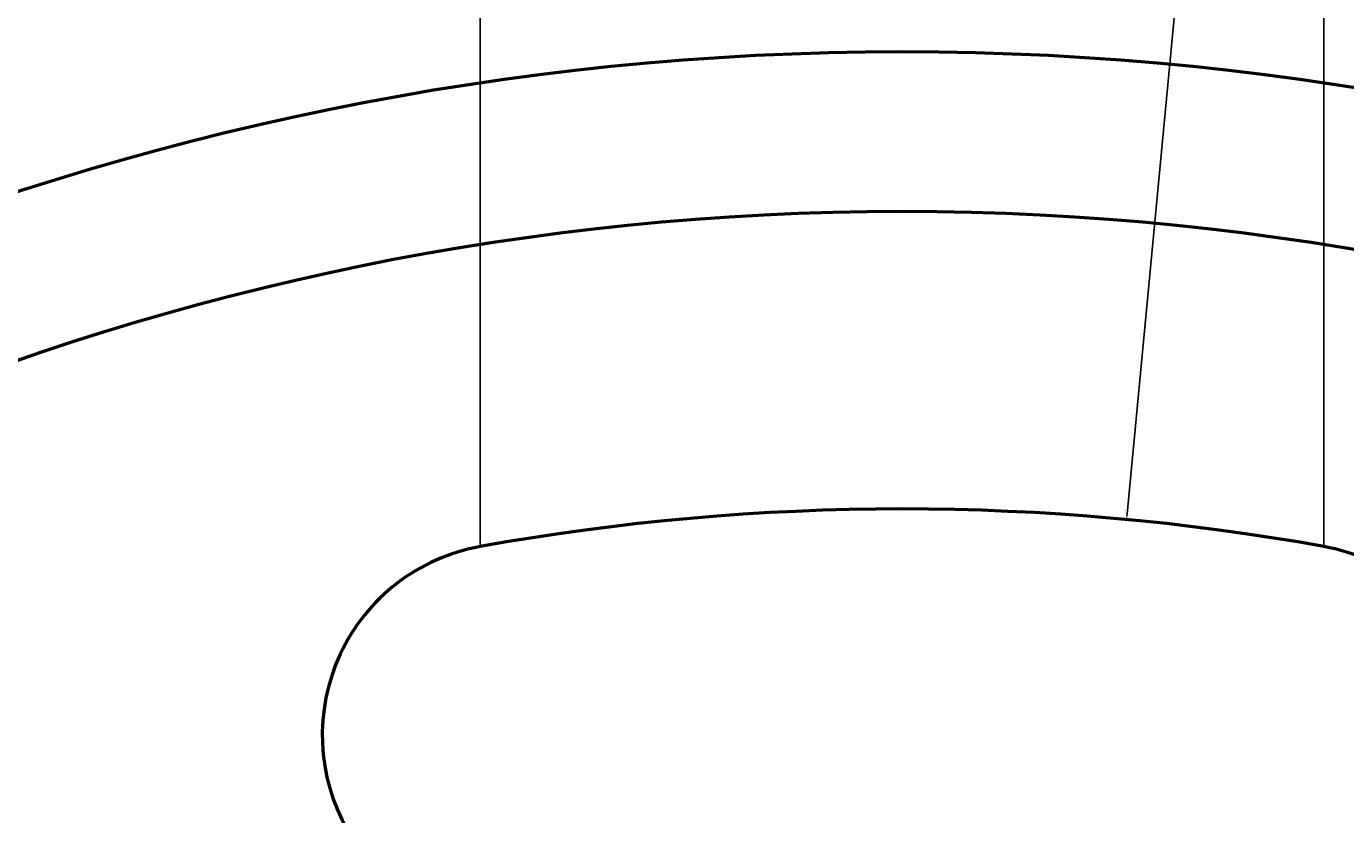
# Model space of a CAD drawing. Units: inches. Extents: x -99 to 284, y -92 to 134.
# Tile 9 of 16: x 5 to 46, y 80 to 105. Entities that reach past the tile are written whole.
import ezdxf

# ---------------------------------------------------------------- set-up
doc = ezdxf.new("R2010")
doc.units = ezdxf.units.IN
doc.header["$MEASUREMENT"] = 0
doc.layers.add('M-DIMS', color=2, linetype='Continuous', lineweight=18)
doc.layers.add('M-OUTL', color=7, linetype='Continuous', lineweight=50)
doc.styles.get("Standard").update_dxf_attribs({"font": 'arial.ttf'})
doc.dimstyles.get("Standard").update_dxf_attribs({"dimtxt": 0.18, "dimasz": 0.18, "dimexe": 0.18, "dimexo": 0.0625, "dimgap": 0.09, "dimtad": 0, "dimtih": 1, "dimtoh": 1, "dimdec": 4, "dimzin": 0, "dimdsep": 46, "dimtxsty": 'Standard', "dimcen": 0.09, "dimadec": 0, "dimazin": 0, "dimtfac": 1, "dimtdec": 4, "dimtofl": 0, "dimtmove": 0, "dimatfit": 3, "dimfxl": 1, "dimtolj": 1, "dimtzin": 0, "dimarcsym": 0})

# ---------------------------------------------------------------- blocks, each defined once
blk = doc.blocks.new('*U1')
for p, q in [((-5.205, -13.52), (-17.34, 7.646)), ((5.205, -13.52), (17.34, 7.646))]:
    blk.add_line(p, q)
for centre, start, end in [((-12.135, 10.63), 100.177, 209.8264), ((12.135, 10.63), 330.1736, 79.823), ((0, -10.536), 209.8264, 330.1736)]:
    blk.add_arc(centre, 6, start, end)
blk = doc.blocks.new('*U2')
at = {"layer": 'M-OUTL', "color": 0, "linetype": 'ByBlock', "lineweight": -2, "transparency": 16777216}
blk.add_blockref('*U1', (31.976, 71.823), dxfattribs=at)
blk = doc.blocks.new('*D10')
at = {"layer": 'Defpoints', "color": 0, "transparency": 16777216}
for p in [(45.172, 120.204), (18.781, 88.36), (45.172, 88.36)]:
    blk.add_point(p, dxfattribs=at)
at = {"layer": 'M-DIMS', "color": 0, "lineweight": -2, "transparency": 16777216}
for p, q in [((18.781, 88.422), (18.781, 120.384)), ((18.961, 120.204), (31.581, 120.204)), ((44.992, 120.204), (32.372, 120.204)), ((45.172, 88.422), (45.172, 120.384))]:
    blk.add_line(p, q, dxfattribs=at)
at = {"layer": 'M-DIMS', "color": 0, "transparency": 16777216}
for points in [[(18.961, 120.234), (18.961, 120.174), (18.781, 120.204)], [(44.992, 120.234), (44.992, 120.174), (45.172, 120.204)]]:
    blk.add_solid(points, dxfattribs=at)
at = {"layer": 'M-DIMS', "color": 0, "transparency": 16777216, "insert": (31.976, 120.204), "char_height": 0.18, "attachment_point": 5}
blk.add_mtext('\\A1;26.39', dxfattribs=at)
blk = doc.blocks.new('*D22')
at = {"layer": 'Defpoints', "color": 0, "transparency": 16777216}
for p in [(39, 89.203), (31.976, 14.854)]:
    blk.add_point(p, dxfattribs=at)
at = {"layer": 'M-DIMS', "color": 0, "lineweight": -2, "transparency": 16777216}
for p, q in [((43.215, 133.813), (39.017, 89.383)), ((43.395, 133.813), (43.215, 133.813)), ((31.976, 14.764), (31.976, 14.944)), ((31.886, 14.854), (32.066, 14.854))]:
    blk.add_line(p, q, dxfattribs=at)
at = {"layer": 'M-DIMS', "color": 0, "transparency": 16777216}
blk.add_solid([(38.987, 89.385), (39.047, 89.38), (39, 89.203)], dxfattribs=at)
at = {"layer": 'M-DIMS', "color": 0, "transparency": 16777216, "insert": (44.068, 133.813), "char_height": 0.18, "attachment_point": 5}
blk.add_mtext('\\A1;5X R74.68', dxfattribs=at)

msp = doc.modelspace()

# ---------------------------------------------------------------- linework, layer by layer
at = {"layer": 'M-OUTL'}
for radius in [89, 84]:
    msp.add_circle((31.9765, 14.8539), radius, dxfattribs=at)
msp.add_arc((31.9765, 14.8539), 74.6806, 79.823035, 100.176965, dxfattribs=at)

# ---------------------------------------------------------------- block references
msp.add_blockref('*U2', (0, 0), dxfattribs=at)

# ---------------------------------------------------------------- dimensions: what is measured, and where the dimension line sits
at = {"layer": 'M-DIMS'}
dim = msp.add_radius_dim(center=(31.9765, 14.8539), mpoint=(39.0003, 89.2035), text='5X <>', dimstyle='Standard', override={"dimdec": 2, "dimlfac": 1, "dimrnd": 0, "dimzin": 0, "dimdsep": 46, "dimlunit": 2}, dxfattribs=at)
dim.commit()
dim.dimension.update_dxf_attribs({"geometry": '*D22', "text_midpoint": (44.068, 133.8132), "dimtype": 164})
dim = msp.add_linear_dim(base=(45.1717, 120.2039), p1=(18.7812, 88.3595), p2=(45.1717, 88.3595), dimstyle='Standard', override={"dimdec": 2, "dimlfac": 1, "dimrnd": 0, "dimzin": 0, "dimdsep": 46, "dimlunit": 2}, dxfattribs=at)
dim.commit()
dim.dimension.update_dxf_attribs({"geometry": '*D10', "text_midpoint": (31.9765, 120.2039)})

doc.saveas('drawing.dxf')
